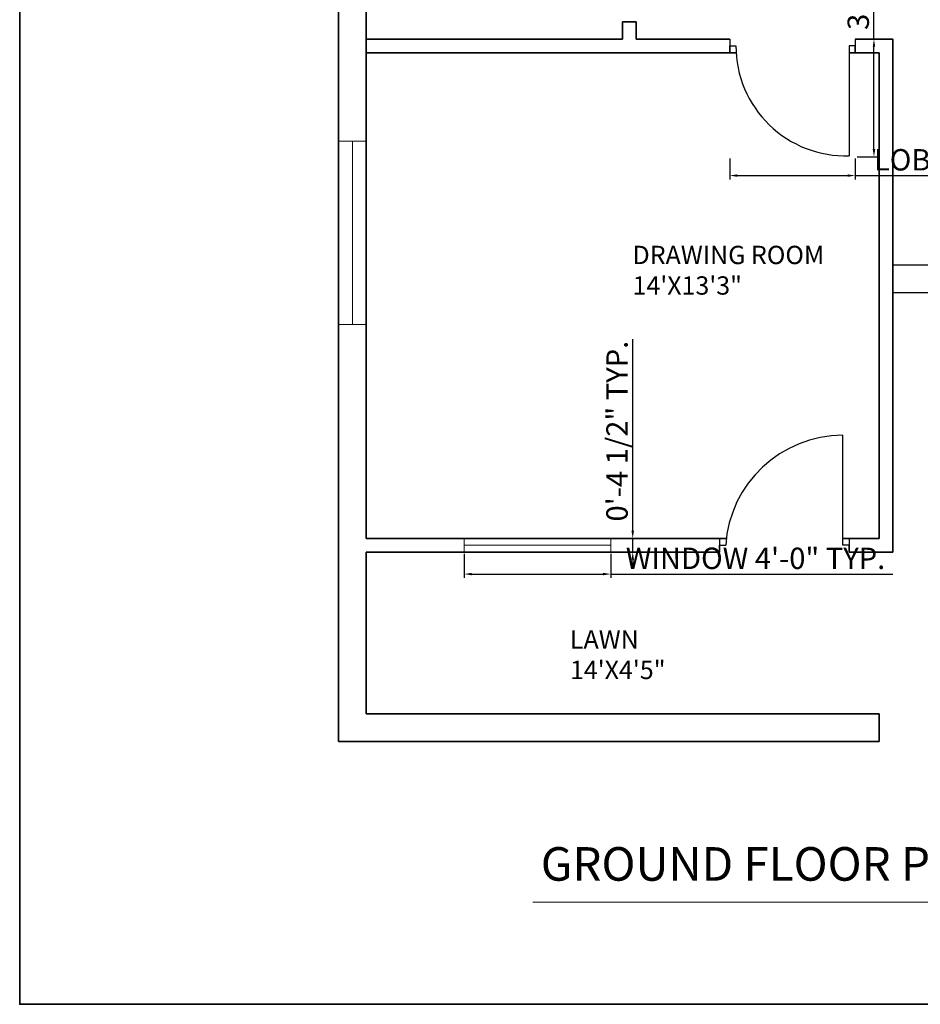
# Model space of a CAD drawing. Units: inches. Extents: x 1863 to 2938, y 1238 to 2492.
# Tile 1 of 12: x 1863 to 2158, y 1253 to 1576. Entities that reach past the tile are written whole.
import ezdxf

# ---------------------------------------------------------------- set-up
doc = ezdxf.new("R2010")
doc.units = ezdxf.units.IN
for name, color, linetype, lineweight in [('A-ANNO-DIMS', 2, 'Continuous', 18), ('A-ANNO-TEXT', 7, 'Continuous', 18), ('A-ANNO-TTLB', 7, 'Continuous', 35), ('A-AREA-IDEN', 7, 'Continuous', 18), ('A-DOOR', 3, 'Continuous', 25), ('A-FLOR-STRS', 7, 'Continuous', 25), ('A-GLAZ', 4, 'Continuous', 18), ('A-WALL', 7, 'Continuous', 35)]:
    doc.layers.add(name, color=color, linetype=linetype, lineweight=lineweight)
doc.styles.get("Standard").update_dxf_attribs({"font": 'arial.ttf'})
doc.dimstyles.new('ISO-25', dxfattribs={"dimtxt": 7, "dimasz": 2.5, "dimexe": 1.25, "dimexo": 0.625, "dimtad": 1, "dimdec": 0, "dimlunit": 3, "dimtxsty": 'Standard', "dimcen": 2.5, "dimadec": 0, "dimazin": 0, "dimtfac": 1, "dimtdec": 0, "dimtmove": 0, "dimatfit": 3, "dimfxl": 1, "dimarcsym": 0})

# ---------------------------------------------------------------- blocks, each defined once
blk = doc.blocks.new('DOOR-36-ENTRY')
for p, q in [((40.4, 2.25), (40.4, 38.25)), ((0, 4.5), (0, 0)), ((42.4, 4.5), (42.4, 0)), ((0, 0), (0, 2.25)), ((0, 2.25), (2, 2.25)), ((42.4, 2.25), (40.4, 2.25)), ((42.4, 0), (42.4, 2.25))]:
    blk.add_line(p, q)
blk.add_arc((40.4, -0.23), 38.48, 90, 176.3006)
blk = doc.blocks.new('DOOR-36-DRAWING')
for p, q in [((0, 38.27), (0, 33.77)), ((0, 33.77), (0, 36.02)), ((0, 36.02), (2, 36.02)), ((41.07, 36.02), (39.07, 36.02)), ((39.07, 36.02), (39.07, 0.02)), ((41.07, 38.27), (41.07, 33.77)), ((41.07, 33.77), (41.07, 36.02))]:
    blk.add_line(p, q)
blk.add_arc((38.02, 36.02), 36.02, 180, 271.6777)
blk = doc.blocks.new('WIN-48')
for p, q in [((0, 4.5), (0, 0)), ((48, 2.25), (48, 4.5)), ((48, 4.5), (48, 0)), ((0, 0), (0, 2.25)), ((0, 2.25), (48, 2.25))]:
    blk.add_line(p, q)
blk = doc.blocks.new('WIN-60')
for p, q in [((0, 60), (9, 60)), ((9, 60), (4.5, 60)), ((4.5, 60), (4.5, 0)), ((4.5, 0), (0, 0)), ((0, 0), (9, 0))]:
    blk.add_line(p, q)
blk = doc.blocks.new('*D28')
at = {"layer": 'A-ANNO-DIMS', "color": 0, "lineweight": -2, "transparency": 16777216}
for p, q in [((2008.76, 1400.94), (2008.76, 1393.11)), ((2056.76, 1400.94), (2056.76, 1393.11)), ((2011.26, 1394.36), (2054.26, 1394.36)), ((2056.76, 1394.36), (2149.09, 1394.36))]:
    blk.add_line(p, q, dxfattribs=at)
at = {"layer": 'A-ANNO-DIMS', "color": 0, "transparency": 16777216}
for points in [[(2011.26, 1394.78), (2011.26, 1393.95), (2008.76, 1394.36)], [(2054.26, 1394.78), (2054.26, 1393.95), (2056.76, 1394.36)]]:
    blk.add_solid(points, dxfattribs=at)
at = {"layer": 'Defpoints', "color": 0, "transparency": 16777216}
for p in [(2008.76, 1401.56), (2056.76, 1401.56), (2056.76, 1394.36)]:
    blk.add_point(p, dxfattribs=at)
at = {"layer": 'A-ANNO-DIMS', "color": 0, "transparency": 16777216, "insert": (2104.18, 1398.61), "char_height": 7, "attachment_point": 5}
blk.add_mtext('WINDOW 4\'-0" TYP.', dxfattribs=at)
blk = doc.blocks.new('*D29')
at = {"layer": 'A-ANNO-DIMS', "color": 0, "lineweight": -2, "transparency": 16777216}
for p, q in [((2063.96, 1408.56), (2063.96, 1471.29)), ((2057.39, 1406.06), (2065.21, 1406.06)), ((2063.96, 1401.56), (2063.96, 1406.06)), ((2057.39, 1401.56), (2065.21, 1401.56)), ((2063.96, 1399.06), (2063.96, 1396.56))]:
    blk.add_line(p, q, dxfattribs=at)
at = {"layer": 'A-ANNO-DIMS', "color": 0, "transparency": 16777216}
for points in [[(2063.55, 1408.56), (2064.38, 1408.56), (2063.96, 1406.06)], [(2063.55, 1399.06), (2064.38, 1399.06), (2063.96, 1401.56)]]:
    blk.add_solid(points, dxfattribs=at)
at = {"layer": 'Defpoints', "color": 0, "transparency": 16777216}
for p in [(2056.76, 1406.06), (2063.96, 1406.06), (2056.76, 1401.56)]:
    blk.add_point(p, dxfattribs=at)
at = {"layer": 'A-ANNO-DIMS', "color": 0, "transparency": 16777216, "insert": (2059.72, 1441.18), "char_height": 7, "attachment_point": 5, "rotation": 90}
blk.add_mtext('0\'-4 1/2" TYP.', dxfattribs=at)
blk = doc.blocks.new('*D56')
at = {"layer": 'A-ANNO-DIMS', "color": 0, "lineweight": -2, "transparency": 16777216}
for p, q in [((2095.74, 1530.4), (2095.74, 1523.62)), ((2136.81, 1530.4), (2136.81, 1523.62)), ((2098.24, 1524.87), (2134.31, 1524.87)), ((2136.81, 1524.87), (2250.3, 1524.87))]:
    blk.add_line(p, q, dxfattribs=at)
at = {"layer": 'A-ANNO-DIMS', "color": 0, "transparency": 16777216}
for points in [[(2098.24, 1525.28), (2098.24, 1524.45), (2095.74, 1524.87)], [(2134.31, 1525.28), (2134.31, 1524.45), (2136.81, 1524.87)]]:
    blk.add_solid(points, dxfattribs=at)
at = {"layer": 'Defpoints', "color": 0, "transparency": 16777216}
for p in [(2095.74, 1531.03), (2136.81, 1531.03), (2136.81, 1524.87)]:
    blk.add_point(p, dxfattribs=at)
at = {"layer": 'A-ANNO-DIMS', "color": 0, "transparency": 16777216, "insert": (2194.8, 1529.12), "char_height": 7, "attachment_point": 5}
blk.add_mtext('LOBBY DOOR 3\'-5" TYP.', dxfattribs=at)
blk = doc.blocks.new('*D57')
at = {"layer": 'A-ANNO-DIMS', "color": 0, "lineweight": -2, "transparency": 16777216}
for p, q in [((2142.97, 1569.56), (2142.97, 1632.29)), ((2137.43, 1569.56), (2144.22, 1569.56)), ((2142.97, 1533.53), (2142.97, 1567.06)), ((2137.43, 1531.03), (2144.22, 1531.03))]:
    blk.add_line(p, q, dxfattribs=at)
at = {"layer": 'A-ANNO-DIMS', "color": 0, "transparency": 16777216}
for points in [[(2142.55, 1567.06), (2143.38, 1567.06), (2142.97, 1569.56)], [(2142.55, 1533.53), (2143.38, 1533.53), (2142.97, 1531.03)]]:
    blk.add_solid(points, dxfattribs=at)
at = {"layer": 'Defpoints', "color": 0, "transparency": 16777216}
for p in [(2136.81, 1569.56), (2142.97, 1569.56), (2136.81, 1531.03)]:
    blk.add_point(p, dxfattribs=at)
at = {"layer": 'A-ANNO-DIMS', "color": 0, "transparency": 16777216, "insert": (2138.72, 1602.17), "char_height": 7, "attachment_point": 5, "rotation": 90}
blk.add_mtext('3\'-2 1/2" TYP.', dxfattribs=at)

msp = doc.modelspace()

# ---------------------------------------------------------------- linework, layer by layer
at = {"layer": 'A-ANNO-TEXT'}
msp.add_line((2031.3, 1286.87), (2208.05, 1286.87), dxfattribs=at)
at = {"layer": 'A-ANNO-TTLB'}
msp.add_lwpolyline([(1863.2, 2492.19), (2938.41, 2492.19), (2938.41, 1253.47), (1863.2, 1253.47)], close=True, dxfattribs=at)
at = {"layer": 'A-FLOR-STRS'}
for p, q in [((2181.02, 1495.56), (2149.14, 1495.56)), ((2149.14, 1495.56), (2149.14, 1486.56)), ((2149.14, 1486.56), (2181.02, 1486.56))]:
    msp.add_line(p, q, dxfattribs=at)
at = {"layer": 'A-WALL'}
for p, q in [((1967.64, 2076.56), (1967.64, 1339.56)), ((1967.64, 2076.56), (1967.64, 1339.56)), ((1976.64, 1622.06), (1976.64, 1406.06)), ((2060.64, 1575.26), (2065.14, 1575.26)), ((2060.64, 1575.26), (2060.64, 1569.56)), ((2065.14, 1575.26), (2065.14, 1569.56)), ((1976.64, 1569.56), (2060.64, 1569.56)), ((2095.74, 1569.56), (2065.14, 1569.56)), ((2144.64, 1569.56), (2136.81, 1569.56)), ((2144.64, 1569.56), (2149.14, 1569.56)), ((2149.14, 1569.56), (2149.14, 1495.56)), ((1976.64, 1565.06), (2060.64, 1565.06)), ((2060.64, 1565.06), (2065.14, 1565.06)), ((2065.14, 1565.06), (2097.81, 1565.06)), ((2134.81, 1565.06), (2144.64, 1565.06)), ((2144.64, 1565.06), (2144.64, 1406.06)), ((2149.14, 1495.56), (2149.14, 1401.56)), ((1976.64, 1406.06), (2094.62, 1406.06)), ((2132.81, 1406.06), (2144.64, 1406.06)), ((1976.64, 1401.56), (2092.4, 1401.56)), ((1976.64, 1401.56), (1976.64, 1348.56)), ((2134.81, 1401.56), (2144.64, 1401.56)), ((2149.14, 1401.56), (2144.64, 1401.56)), ((1976.64, 1348.56), (2144.64, 1348.56)), ((2144.64, 1348.56), (2144.64, 1339.56)), ((1967.64, 1339.56), (2144.64, 1339.56))]:
    msp.add_line(p, q, dxfattribs=at)

# ---------------------------------------------------------------- block references
at = {"layer": 'A-DOOR'}
for name, p in [('DOOR-36-DRAWING', (2095.74, 1531.3)), ('DOOR-36-ENTRY', (2092.4, 1401.56))]:
    msp.add_blockref(name, p, dxfattribs=at)
at = {"layer": 'A-GLAZ'}
for name, p in [('WIN-60', (1967.64, 1476.09)), ('WIN-48', (2008.76, 1401.56))]:
    msp.add_blockref(name, p, dxfattribs=at)

# ---------------------------------------------------------------- texts
at = {"layer": 'A-ANNO-TEXT', "insert": (2033.86, 1304.94), "char_height": 11, "attachment_point": 1}
msp.add_mtext_dynamic_manual_height_columns('GROUND FLOOR PLAN', width=285.9914, gutter_width=12.5, heights=[0], dxfattribs=at)
at = {"layer": 'A-AREA-IDEN', "char_height": 6, "attachment_point": 1}
for s, width, insert in [('DRAWING ROOM\\P14\'X13\'3"', 147.6504, (2063.9, 1501.87)), ('LAWN\\P14\'X4\'5"', 112.1146, (2043.41, 1375.98))]:
    msp.add_mtext_dynamic_manual_height_columns(s, width=width, gutter_width=12.5, heights=[0], dxfattribs=dict(at, insert=insert))

# ---------------------------------------------------------------- dimensions: what is measured, and where the dimension line sits
at = {"layer": 'A-ANNO-DIMS'}
for base, p1, p2, picture, middle in [((2142.97, 1569.56), (2136.81, 1531.03), (2136.81, 1569.56), '*D57', (2138.72, 1602.17)), ((2063.96, 1406.06), (2056.76, 1401.56), (2056.76, 1406.06), '*D29', (2059.72, 1441.18))]:
    dim = msp.add_linear_dim(base=base, p1=p1, p2=p2, angle=90, text='<> TYP.', dimstyle='ISO-25', override={"dimdec": 1, "dimlfac": 1, "dimrnd": 0, "dimzin": 1, "dimdsep": 46, "dimlunit": 4, "dimfrac": 2}, dxfattribs=at)
    dim.commit()
    dim.dimension.update_dxf_attribs({"geometry": picture, "text_midpoint": middle})
for base, p1, p2, text, picture, middle in [((2136.81, 1524.87), (2095.74, 1531.03), (2136.81, 1531.03), 'LOBBY DOOR <> TYP.', '*D56', (2194.8, 1529.12)), ((2056.76, 1394.36), (2008.76, 1401.56), (2056.76, 1401.56), 'WINDOW <> TYP.', '*D28', (2104.18, 1398.61))]:
    dim = msp.add_linear_dim(base=base, p1=p1, p2=p2, text=text, dimstyle='ISO-25', override={"dimdec": 1, "dimlfac": 1, "dimrnd": 0, "dimzin": 1, "dimdsep": 46, "dimlunit": 4, "dimfrac": 2}, dxfattribs=at)
    dim.commit()
    dim.dimension.update_dxf_attribs({"geometry": picture, "text_midpoint": middle})

doc.saveas('drawing.dxf')
